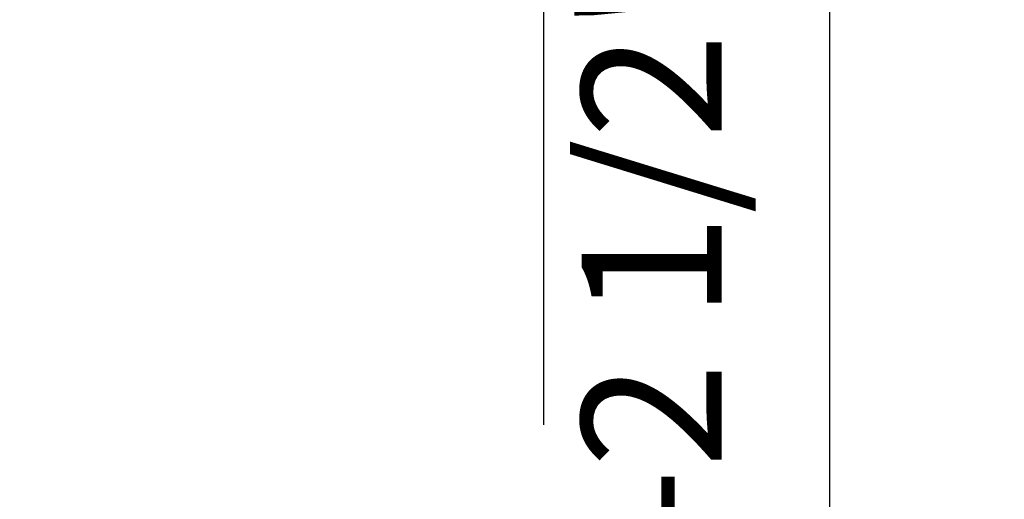
# Model space of a CAD drawing. Units: millimetres. Extents: x 7894 to 8038, y 6851 to 6951.
# Tile 42 of 49: x 7968.188 to 7975.227, y 6928.457 to 6931.885. Entities that reach past the tile are written whole.
import ezdxf

# ---------------------------------------------------------------- set-up
doc = ezdxf.new("R2010")
doc.units = ezdxf.units.MM
doc.layers.add('A-ANNO-DIMS', color=2, linetype='Continuous', lineweight=18)
doc.styles.get("Standard").update_dxf_attribs({"font": 'arial.ttf'})
doc.dimstyles.new('ISO-25', dxfattribs={"dimtxt": 1, "dimasz": 1, "dimexe": 1.25, "dimexo": 0.625, "dimtad": 1, "dimdec": 0, "dimlunit": 4, "dimtxsty": 'Standard', "dimcen": 2.5, "dimclrt": 1, "dimadec": 0, "dimazin": 0, "dimtfac": 1, "dimtdec": 0, "dimtmove": 0, "dimatfit": 3, "dimfxl": 1, "dimarcsym": 0})

# ---------------------------------------------------------------- blocks, each defined once
blk = doc.blocks.new('*D23')
at = {"layer": 'A-ANNO-DIMS', "color": 0, "lineweight": -2, "transparency": 16777216}
for p, q in [((7940.0888, 6907.098), (7940.0888, 6947.7928)), ((7971.9356, 6928.989), (7971.9356, 6947.7928)), ((7941.0888, 6946.5428), (7970.9356, 6946.5428))]:
    blk.add_line(p, q, dxfattribs=at)
at = {"layer": 'A-ANNO-DIMS', "color": 0, "transparency": 16777216}
for points in [[(7941.0888, 6946.7095), (7941.0888, 6946.3762), (7940.0888, 6946.5428)], [(7970.9356, 6946.7095), (7970.9356, 6946.3762), (7971.9356, 6946.5428)]]:
    blk.add_solid(points, dxfattribs=at)
at = {"layer": 'Defpoints', "color": 0, "transparency": 16777216}
for p in [(7971.9356, 6946.5428), (7971.9356, 6928.364), (7940.0888, 6906.473)]:
    blk.add_point(p, dxfattribs=at)
at = {"layer": 'A-ANNO-DIMS', "color": 1, "transparency": 16777216, "insert": (7956.0122, 6947.6784), "char_height": 1, "attachment_point": 5}
blk.add_mtext('2\'-8"', dxfattribs=at)
blk = doc.blocks.new('*D28')
at = {"layer": 'A-ANNO-DIMS', "color": 0, "lineweight": -2, "transparency": 16777216}
for p, q in [((7960.8854, 6936.8804), (7975.2272, 6936.8804)), ((7973.9772, 6935.8804), (7973.9772, 6923.6283)), ((7971.8421, 6922.6283), (7975.2272, 6922.6283))]:
    blk.add_line(p, q, dxfattribs=at)
at = {"layer": 'A-ANNO-DIMS', "color": 0, "transparency": 16777216}
for points in [[(7973.8105, 6935.8804), (7974.1439, 6935.8804), (7973.9772, 6936.8804)], [(7973.8105, 6923.6283), (7974.1439, 6923.6283), (7973.9772, 6922.6283)]]:
    blk.add_solid(points, dxfattribs=at)
at = {"layer": 'Defpoints', "color": 0, "transparency": 16777216}
for p in [(7960.2604, 6936.8804), (7971.2171, 6922.6283), (7973.9772, 6922.6283)]:
    blk.add_point(p, dxfattribs=at)
at = {"layer": 'A-ANNO-DIMS', "color": 1, "transparency": 16777216, "insert": (7972.8351, 6929.7543), "char_height": 1, "attachment_point": 5, "rotation": 90}
blk.add_mtext('1\'-2 1/2"', dxfattribs=at)

msp = doc.modelspace()

# ---------------------------------------------------------------- dimensions: what is measured, and where the dimension line sits
at = {"layer": 'A-ANNO-DIMS'}
dim = msp.add_linear_dim(base=(7971.9356, 6946.5428), p1=(7940.0888, 6906.473), p2=(7971.9356, 6928.364), dimstyle='ISO-25', override={"dimdec": 1, "dimlfac": 1, "dimrnd": 0, "dimzin": 1, "dimdsep": 46, "dimlunit": 4, "dimfrac": 2}, dxfattribs=at)
dim.commit()
dim.dimension.update_dxf_attribs({"geometry": '*D23', "text_midpoint": (7956.0122, 6947.6784)})
dim = msp.add_linear_dim(base=(7973.9772, 6922.6283), p1=(7960.2604, 6936.8804), p2=(7971.2171, 6922.6283), angle=90, dimstyle='ISO-25', override={"dimdec": 1, "dimlfac": 1, "dimrnd": 0, "dimzin": 1, "dimdsep": 46, "dimlunit": 4, "dimfrac": 2}, dxfattribs=at)
dim.commit()
dim.dimension.update_dxf_attribs({"geometry": '*D28', "text_midpoint": (7972.8351, 6929.7543)})

doc.saveas('drawing.dxf')
